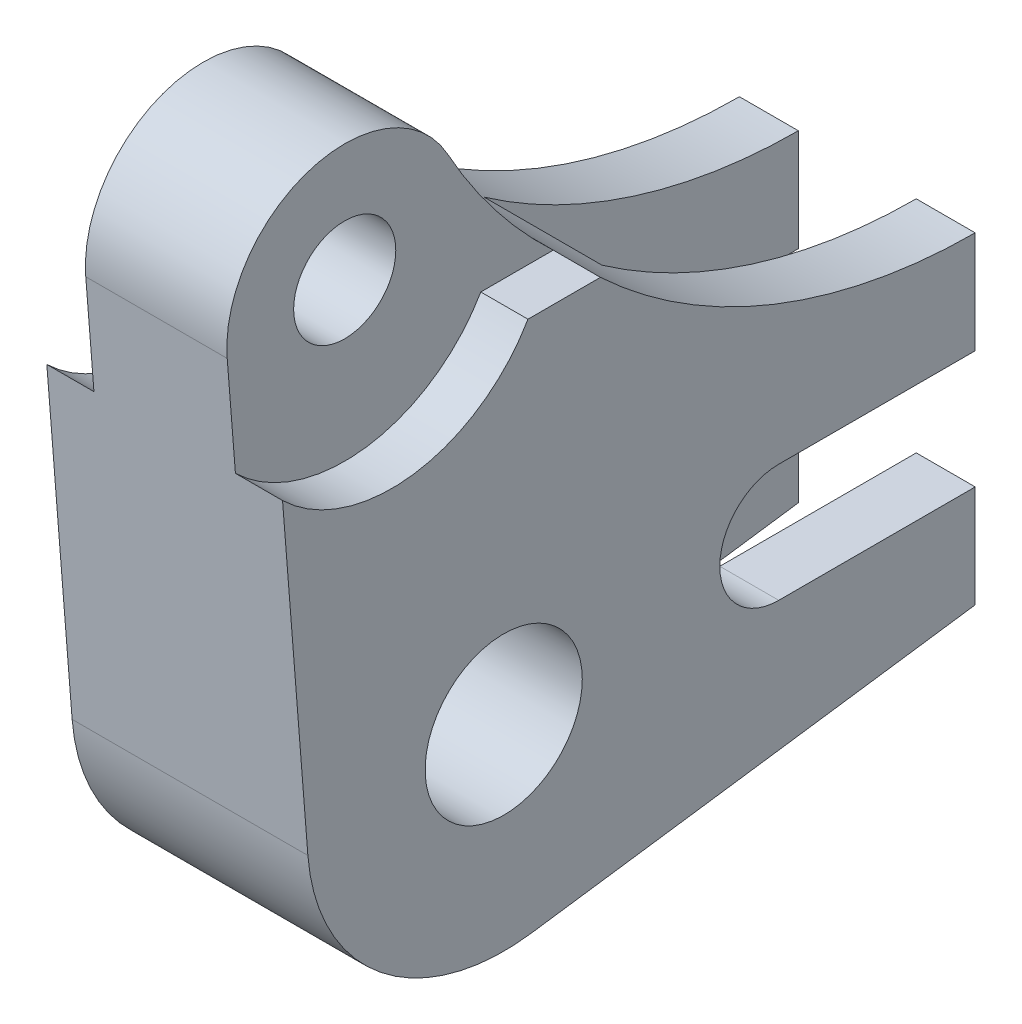
ISO-10303-21;
HEADER;
FILE_DESCRIPTION(('STEP AP214'),'2;1');
FILE_NAME('part.step','',(''),(''),'','','');
FILE_SCHEMA(('AUTOMOTIVE_DESIGN { 1 0 10303 214 1 1 1 1 }'));
ENDSEC;
DATA;
#1=APPLICATION_CONTEXT('core data for automotive mechanical design processes');
#2=APPLICATION_PROTOCOL_DEFINITION('international standard','automotive_design',2000,#1);
#3=PRODUCT_CONTEXT('',#1,'mechanical');
#4=PRODUCT('Part','Part','',(#3));
#5=PRODUCT_RELATED_PRODUCT_CATEGORY('part','',(#4));
#6=PRODUCT_DEFINITION_FORMATION('','',#4);
#7=PRODUCT_DEFINITION_CONTEXT('part definition',#1,'design');
#8=PRODUCT_DEFINITION('design','',#6,#7);
#9=PRODUCT_DEFINITION_SHAPE('','',#8);
#10=(LENGTH_UNIT() NAMED_UNIT(*) SI_UNIT(.MILLI.,.METRE.));
#11=(NAMED_UNIT(*) PLANE_ANGLE_UNIT() SI_UNIT($,.RADIAN.));
#12=(NAMED_UNIT(*) SI_UNIT($,.STERADIAN.) SOLID_ANGLE_UNIT());
#13=UNCERTAINTY_MEASURE_WITH_UNIT(LENGTH_MEASURE(1.E-05),#10,'distance_accuracy_value','');
#14=(GEOMETRIC_REPRESENTATION_CONTEXT(3) GLOBAL_UNCERTAINTY_ASSIGNED_CONTEXT((#13)) GLOBAL_UNIT_ASSIGNED_CONTEXT((#10,
#11,#12)) REPRESENTATION_CONTEXT('',''));
#15=CARTESIAN_POINT('',(0.,0.,0.));
#16=DIRECTION('',(0.,0.,1.));
#17=DIRECTION('',(1.,0.,0.));
#18=AXIS2_PLACEMENT_3D('',#15,#16,#17);
#19=CARTESIAN_POINT('',(15.,-3.81323923082236,-60.));
#20=DIRECTION('',(0.,0.,1.));
#21=DIRECTION('',(1.,0.,0.));
#22=AXIS2_PLACEMENT_3D('',#19,#20,#21);
#23=PLANE('',#22);
#24=DIRECTION('',(0.,-1.,0.));
#25=VECTOR('',#24,1.);
#26=CARTESIAN_POINT('',(7.5,68.1259204458987,-60.));
#27=LINE('',#26,#25);
#28=CARTESIAN_POINT('',(7.5,-3.81323923082236,-60.));
#29=VERTEX_POINT('',#28);
#30=CARTESIAN_POINT('',(7.5,-16.8132392308223,-60.));
#31=VERTEX_POINT('',#30);
#32=EDGE_CURVE('E199',#29,#31,#27,.T.);
#33=ORIENTED_EDGE('',*,*,#32,.F.);
#34=DIRECTION('',(-1.,0.,0.));
#35=VECTOR('',#34,1.);
#36=CARTESIAN_POINT('',(15.,-3.81323923082236,-60.));
#37=LINE('',#36,#35);
#38=CARTESIAN_POINT('',(15.,-3.81323923082236,-60.));
#39=VERTEX_POINT('',#38);
#40=EDGE_CURVE('E361',#39,#29,#37,.T.);
#41=ORIENTED_EDGE('',*,*,#40,.F.);
#42=DIRECTION('',(0.,1.,0.));
#43=VECTOR('',#42,1.);
#44=CARTESIAN_POINT('',(15.,-3.81323923082236,-60.));
#45=LINE('',#44,#43);
#46=CARTESIAN_POINT('',(15.,-16.8132392308224,-60.));
#47=VERTEX_POINT('',#46);
#48=EDGE_CURVE('E296',#47,#39,#45,.T.);
#49=ORIENTED_EDGE('',*,*,#48,.F.);
#50=DIRECTION('',(-1.,0.,0.));
#51=VECTOR('',#50,1.);
#52=CARTESIAN_POINT('',(15.,-16.8132392308224,-60.));
#53=LINE('',#52,#51);
#54=EDGE_CURVE('E370',#47,#31,#53,.T.);
#55=ORIENTED_EDGE('',*,*,#54,.T.);
#56=EDGE_LOOP('',(#33,#41,#49,#55));
#57=FACE_BOUND('',#56,.T.);
#58=ADVANCED_FACE('F39',(#57),#23,.F.);
#59=CARTESIAN_POINT('',(15.,24.1867607691776,-60.));
#60=DIRECTION('',(0.,0.,1.));
#61=DIRECTION('',(0.,-1.,0.));
#62=AXIS2_PLACEMENT_3D('',#59,#60,#61);
#63=PLANE('',#62);
#64=CARTESIAN_POINT('',(7.5,24.1867607691776,-60.));
#65=VERTEX_POINT('',#64);
#66=CARTESIAN_POINT('',(7.5,11.1867607691776,-60.));
#67=VERTEX_POINT('',#66);
#68=EDGE_CURVE('E214',#65,#67,#27,.T.);
#69=ORIENTED_EDGE('',*,*,#68,.F.);
#70=DIRECTION('',(-1.,0.,0.));
#71=VECTOR('',#70,1.);
#72=CARTESIAN_POINT('',(15.,24.1867607691776,-60.));
#73=LINE('',#72,#71);
#74=CARTESIAN_POINT('',(15.,24.1867607691776,-60.));
#75=VERTEX_POINT('',#74);
#76=EDGE_CURVE('E350',#75,#65,#73,.T.);
#77=ORIENTED_EDGE('',*,*,#76,.F.);
#78=DIRECTION('',(0.,1.,0.));
#79=VECTOR('',#78,1.);
#80=CARTESIAN_POINT('',(15.,24.1867607691776,-60.));
#81=LINE('',#80,#79);
#82=CARTESIAN_POINT('',(15.,11.1867607691776,-60.));
#83=VERTEX_POINT('',#82);
#84=EDGE_CURVE('E308',#83,#75,#81,.T.);
#85=ORIENTED_EDGE('',*,*,#84,.F.);
#86=DIRECTION('',(-1.,0.,0.));
#87=VECTOR('',#86,1.);
#88=CARTESIAN_POINT('',(15.,11.1867607691776,-60.));
#89=LINE('',#88,#87);
#90=EDGE_CURVE('E353',#83,#67,#89,.T.);
#91=ORIENTED_EDGE('',*,*,#90,.T.);
#92=EDGE_LOOP('',(#69,#77,#85,#91));
#93=FACE_BOUND('',#92,.T.);
#94=ADVANCED_FACE('F379',(#93),#63,.F.);
#95=CARTESIAN_POINT('',(15.,-16.8132392308224,-60.));
#96=DIRECTION('',(0.,0.990268068741571,0.139173100960059));
#97=DIRECTION('',(0.,-0.139173100960059,0.990268068741571));
#98=AXIS2_PLACEMENT_3D('',#95,#96,#97);
#99=PLANE('',#98);
#100=DIRECTION('',(0.,0.139173100960059,-0.990268068741571));
#101=VECTOR('',#100,1.);
#102=CARTESIAN_POINT('',(-7.5,-16.8132392308224,-60.));
#103=LINE('',#102,#101);
#104=CARTESIAN_POINT('',(-7.49999999999999,-22.4348726189177,-20.));
#105=VERTEX_POINT('',#104);
#106=CARTESIAN_POINT('',(-7.5,-16.8132392308223,-60.));
#107=VERTEX_POINT('',#106);
#108=EDGE_CURVE('E219',#105,#107,#103,.T.);
#109=ORIENTED_EDGE('',*,*,#108,.F.);
#110=DIRECTION('',(-1.,0.,0.));
#111=VECTOR('',#110,1.);
#112=CARTESIAN_POINT('',(15.,-22.4348726189177,-20.));
#113=LINE('',#112,#111);
#114=CARTESIAN_POINT('',(7.50000000000001,-22.4348726189177,-20.));
#115=VERTEX_POINT('',#114);
#116=EDGE_CURVE('E202',#115,#105,#113,.T.);
#117=ORIENTED_EDGE('',*,*,#116,.F.);
#118=DIRECTION('',(0.,-0.139173100960059,0.990268068741571));
#119=VECTOR('',#118,1.);
#120=CARTESIAN_POINT('',(7.5,-16.8132392308224,-60.));
#121=LINE('',#120,#119);
#122=EDGE_CURVE('E197',#31,#115,#121,.T.);
#123=ORIENTED_EDGE('',*,*,#122,.F.);
#124=ORIENTED_EDGE('',*,*,#54,.F.);
#125=DIRECTION('',(0.,0.139173100960059,-0.990268068741571));
#126=VECTOR('',#125,1.);
#127=CARTESIAN_POINT('',(15.,-16.8132392308224,-60.));
#128=LINE('',#127,#126);
#129=CARTESIAN_POINT('',(15.,-24.7567017185393,-3.47932752400147));
#130=VERTEX_POINT('',#129);
#131=EDGE_CURVE('E293',#130,#47,#128,.T.);
#132=ORIENTED_EDGE('',*,*,#131,.F.);
#133=DIRECTION('',(-1.,0.,0.));
#134=VECTOR('',#133,1.);
#135=CARTESIAN_POINT('',(15.,-24.7567017185393,-3.47932752400147));
#136=LINE('',#135,#134);
#137=CARTESIAN_POINT('',(-15.,-24.7567017185393,-3.47932752400147));
#138=VERTEX_POINT('',#137);
#139=EDGE_CURVE('E369',#130,#138,#136,.T.);
#140=ORIENTED_EDGE('',*,*,#139,.T.);
#141=DIRECTION('',(0.,0.139173100960059,-0.990268068741571));
#142=VECTOR('',#141,1.);
#143=CARTESIAN_POINT('',(-15.,-16.8132392308224,-60.));
#144=LINE('',#143,#142);
#145=CARTESIAN_POINT('',(-15.,-16.8132392308224,-60.));
#146=VERTEX_POINT('',#145);
#147=EDGE_CURVE('E316',#138,#146,#144,.T.);
#148=ORIENTED_EDGE('',*,*,#147,.T.);
#149=EDGE_CURVE('E368',#107,#146,#53,.T.);
#150=ORIENTED_EDGE('',*,*,#149,.F.);
#151=EDGE_LOOP('',(#109,#117,#123,#124,#132,#140,#148,#150));
#152=FACE_BOUND('',#151,.T.);
#153=ADVANCED_FACE('F217',(#152),#99,.F.);
#154=CARTESIAN_POINT('',(15.,-3.81323923082236,-35.));
#155=DIRECTION('',(0.,-1.,0.));
#156=DIRECTION('',(0.,0.,-1.));
#157=AXIS2_PLACEMENT_3D('',#154,#155,#156);
#158=PLANE('',#157);
#159=DIRECTION('',(0.,0.,1.));
#160=VECTOR('',#159,1.);
#161=CARTESIAN_POINT('',(-7.5,-3.81323923082236,-35.));
#162=LINE('',#161,#160);
#163=CARTESIAN_POINT('',(-7.5,-3.81323923082236,-60.));
#164=VERTEX_POINT('',#163);
#165=CARTESIAN_POINT('',(-7.5,-3.81323923082236,-35.));
#166=VERTEX_POINT('',#165);
#167=EDGE_CURVE('E226',#164,#166,#162,.T.);
#168=ORIENTED_EDGE('',*,*,#167,.F.);
#169=CARTESIAN_POINT('',(-15.,-3.81323923082236,-60.));
#170=VERTEX_POINT('',#169);
#171=EDGE_CURVE('E362',#164,#170,#37,.T.);
#172=ORIENTED_EDGE('',*,*,#171,.T.);
#173=DIRECTION('',(0.,0.,1.));
#174=VECTOR('',#173,1.);
#175=CARTESIAN_POINT('',(-15.,-3.81323923082236,-35.));
#176=LINE('',#175,#174);
#177=CARTESIAN_POINT('',(-15.,-3.81323923082236,-35.));
#178=VERTEX_POINT('',#177);
#179=EDGE_CURVE('E325',#170,#178,#176,.T.);
#180=ORIENTED_EDGE('',*,*,#179,.T.);
#181=DIRECTION('',(-1.,0.,0.));
#182=VECTOR('',#181,1.);
#183=CARTESIAN_POINT('',(15.,-3.81323923082236,-35.));
#184=LINE('',#183,#182);
#185=EDGE_CURVE('E360',#166,#178,#184,.T.);
#186=ORIENTED_EDGE('',*,*,#185,.F.);
#187=EDGE_LOOP('',(#168,#172,#180,#186));
#188=FACE_BOUND('',#187,.T.);
#189=ADVANCED_FACE('F503',(#188),#158,.F.);
#190=DIRECTION('',(0.,0.,-1.));
#191=VECTOR('',#190,1.);
#192=CARTESIAN_POINT('',(7.5,-3.81323923082236,-35.));
#193=LINE('',#192,#191);
#194=CARTESIAN_POINT('',(7.5,-3.81323923082236,-35.));
#195=VERTEX_POINT('',#194);
#196=EDGE_CURVE('E206',#195,#29,#193,.T.);
#197=ORIENTED_EDGE('',*,*,#196,.F.);
#198=CARTESIAN_POINT('',(15.,-3.81323923082236,-35.));
#199=VERTEX_POINT('',#198);
#200=EDGE_CURVE('E356',#199,#195,#184,.T.);
#201=ORIENTED_EDGE('',*,*,#200,.F.);
#202=DIRECTION('',(0.,0.,1.));
#203=VECTOR('',#202,1.);
#204=CARTESIAN_POINT('',(15.,-3.81323923082236,-35.));
#205=LINE('',#204,#203);
#206=EDGE_CURVE('E299',#39,#199,#205,.T.);
#207=ORIENTED_EDGE('',*,*,#206,.F.);
#208=ORIENTED_EDGE('',*,*,#40,.T.);
#209=EDGE_LOOP('',(#197,#201,#207,#208));
#210=FACE_BOUND('',#209,.T.);
#211=ADVANCED_FACE('F414',(#210),#158,.F.);
#212=CARTESIAN_POINT('',(15.,3.68676076917764,-35.));
#213=DIRECTION('',(-1.,0.,0.));
#214=DIRECTION('',(0.,0.,1.));
#215=AXIS2_PLACEMENT_3D('',#212,#213,#214);
#216=CYLINDRICAL_SURFACE('',#215,7.5);
#217=CARTESIAN_POINT('',(-7.5,3.68676076917764,-35.));
#218=DIRECTION('',(1.,0.,0.));
#219=DIRECTION('',(0.,0.,-1.));
#220=AXIS2_PLACEMENT_3D('',#217,#218,#219);
#221=CIRCLE('',#220,7.5);
#222=CARTESIAN_POINT('',(-7.5,11.1867607691776,-35.));
#223=VERTEX_POINT('',#222);
#224=EDGE_CURVE('E224',#166,#223,#221,.F.);
#225=ORIENTED_EDGE('',*,*,#224,.F.);
#226=ORIENTED_EDGE('',*,*,#185,.T.);
#227=CARTESIAN_POINT('',(-15.,3.68676076917764,-35.));
#228=DIRECTION('',(-1.,0.,0.));
#229=DIRECTION('',(0.,0.,-1.));
#230=AXIS2_PLACEMENT_3D('',#227,#228,#229);
#231=CIRCLE('',#230,7.5);
#232=CARTESIAN_POINT('',(-15.,11.1867607691776,-35.));
#233=VERTEX_POINT('',#232);
#234=EDGE_CURVE('E324',#178,#233,#231,.T.);
#235=ORIENTED_EDGE('',*,*,#234,.T.);
#236=DIRECTION('',(-1.,0.,0.));
#237=VECTOR('',#236,1.);
#238=CARTESIAN_POINT('',(15.,11.1867607691776,-35.));
#239=LINE('',#238,#237);
#240=EDGE_CURVE('E352',#223,#233,#239,.T.);
#241=ORIENTED_EDGE('',*,*,#240,.F.);
#242=EDGE_LOOP('',(#225,#226,#235,#241));
#243=FACE_BOUND('',#242,.T.);
#244=ADVANCED_FACE('F499',(#243),#216,.F.);
#245=CARTESIAN_POINT('',(7.5,3.68676076917764,-35.));
#246=DIRECTION('',(-1.,0.,0.));
#247=DIRECTION('',(0.,0.,1.));
#248=AXIS2_PLACEMENT_3D('',#245,#246,#247);
#249=CIRCLE('',#248,7.5);
#250=CARTESIAN_POINT('',(7.5,11.1867607691776,-35.));
#251=VERTEX_POINT('',#250);
#252=EDGE_CURVE('E398',#251,#195,#249,.F.);
#253=ORIENTED_EDGE('',*,*,#252,.F.);
#254=CARTESIAN_POINT('',(15.,11.1867607691776,-35.));
#255=VERTEX_POINT('',#254);
#256=EDGE_CURVE('E354',#255,#251,#239,.T.);
#257=ORIENTED_EDGE('',*,*,#256,.F.);
#258=CARTESIAN_POINT('',(15.,3.68676076917764,-35.));
#259=DIRECTION('',(-1.,0.,0.));
#260=DIRECTION('',(0.,0.,-1.));
#261=AXIS2_PLACEMENT_3D('',#258,#259,#260);
#262=CIRCLE('',#261,7.5);
#263=EDGE_CURVE('E304',#199,#255,#262,.T.);
#264=ORIENTED_EDGE('',*,*,#263,.F.);
#265=ORIENTED_EDGE('',*,*,#200,.T.);
#266=EDGE_LOOP('',(#253,#257,#264,#265));
#267=FACE_BOUND('',#266,.T.);
#268=ADVANCED_FACE('F500',(#267),#216,.F.);
#269=CARTESIAN_POINT('',(15.,11.1867607691776,-60.));
#270=DIRECTION('',(0.,1.,0.));
#271=DIRECTION('',(0.,0.,1.));
#272=AXIS2_PLACEMENT_3D('',#269,#270,#271);
#273=PLANE('',#272);
#274=DIRECTION('',(0.,0.,-1.));
#275=VECTOR('',#274,1.);
#276=CARTESIAN_POINT('',(-7.5,11.1867607691776,-60.));
#277=LINE('',#276,#275);
#278=CARTESIAN_POINT('',(-7.5,11.1867607691776,-60.));
#279=VERTEX_POINT('',#278);
#280=EDGE_CURVE('E222',#223,#279,#277,.T.);
#281=ORIENTED_EDGE('',*,*,#280,.F.);
#282=ORIENTED_EDGE('',*,*,#240,.T.);
#283=DIRECTION('',(0.,0.,-1.));
#284=VECTOR('',#283,1.);
#285=CARTESIAN_POINT('',(-15.,11.1867607691776,-60.));
#286=LINE('',#285,#284);
#287=CARTESIAN_POINT('',(-15.,11.1867607691776,-60.));
#288=VERTEX_POINT('',#287);
#289=EDGE_CURVE('E327',#233,#288,#286,.T.);
#290=ORIENTED_EDGE('',*,*,#289,.T.);
#291=EDGE_CURVE('E348',#279,#288,#89,.T.);
#292=ORIENTED_EDGE('',*,*,#291,.F.);
#293=EDGE_LOOP('',(#281,#282,#290,#292));
#294=FACE_BOUND('',#293,.T.);
#295=ADVANCED_FACE('F438',(#294),#273,.F.);
#296=DIRECTION('',(0.,0.,1.));
#297=VECTOR('',#296,1.);
#298=CARTESIAN_POINT('',(7.5,11.1867607691776,-60.));
#299=LINE('',#298,#297);
#300=EDGE_CURVE('E400',#67,#251,#299,.T.);
#301=ORIENTED_EDGE('',*,*,#300,.F.);
#302=ORIENTED_EDGE('',*,*,#90,.F.);
#303=DIRECTION('',(0.,0.,-1.));
#304=VECTOR('',#303,1.);
#305=CARTESIAN_POINT('',(15.,11.1867607691776,-60.));
#306=LINE('',#305,#304);
#307=EDGE_CURVE('E301',#255,#83,#306,.T.);
#308=ORIENTED_EDGE('',*,*,#307,.F.);
#309=ORIENTED_EDGE('',*,*,#256,.T.);
#310=EDGE_LOOP('',(#301,#302,#308,#309));
#311=FACE_BOUND('',#310,.T.);
#312=ADVANCED_FACE('F399',(#311),#273,.F.);
#313=CARTESIAN_POINT('',(15.,94.1865039901961,-60.1896021927174));
#314=DIRECTION('',(-1.,0.,0.));
#315=DIRECTION('',(0.,0.,1.));
#316=AXIS2_PLACEMENT_3D('',#313,#314,#315);
#317=CYLINDRICAL_SURFACE('',#316,70.);
#318=CARTESIAN_POINT('',(-7.5,94.1865039901961,-60.1896021927174));
#319=DIRECTION('',(1.,0.,0.));
#320=DIRECTION('',(0.,0.,-1.));
#321=AXIS2_PLACEMENT_3D('',#318,#319,#320);
#322=CIRCLE('',#321,70.);
#323=CARTESIAN_POINT('',(-7.5,24.1867607691776,-60.));
#324=VERTEX_POINT('',#323);
#325=CARTESIAN_POINT('',(-7.49999999999999,36.8733652208779,-20.));
#326=VERTEX_POINT('',#325);
#327=EDGE_CURVE('E11',#324,#326,#322,.F.);
#328=ORIENTED_EDGE('',*,*,#327,.F.);
#329=CARTESIAN_POINT('',(-15.,24.1867607691776,-60.));
#330=VERTEX_POINT('',#329);
#331=EDGE_CURVE('E347',#324,#330,#73,.T.);
#332=ORIENTED_EDGE('',*,*,#331,.T.);
#333=CARTESIAN_POINT('',(-15.,94.1865039901961,-60.1896021927174));
#334=DIRECTION('',(-1.,0.,0.));
#335=DIRECTION('',(0.,0.,-1.));
#336=AXIS2_PLACEMENT_3D('',#333,#334,#335);
#337=CIRCLE('',#336,70.);
#338=CARTESIAN_POINT('',(-15.,43.1259204458988,-12.3062354761233));
#339=VERTEX_POINT('',#338);
#340=EDGE_CURVE('E331',#330,#339,#337,.T.);
#341=ORIENTED_EDGE('',*,*,#340,.T.);
#342=DIRECTION('',(-1.,0.,0.));
#343=VECTOR('',#342,1.);
#344=CARTESIAN_POINT('',(-9.,43.1259204458988,-12.3062354761233));
#345=LINE('',#344,#343);
#346=CARTESIAN_POINT('',(-9.,43.1259204458988,-12.3062354761233));
#347=VERTEX_POINT('',#346);
#348=EDGE_CURVE('E255',#347,#339,#345,.T.);
#349=ORIENTED_EDGE('',*,*,#348,.F.);
#350=CARTESIAN_POINT('',(-9.,94.1865039901961,-60.1896021927174));
#351=DIRECTION('',(-1.,0.,0.));
#352=DIRECTION('',(0.,0.,-1.));
#353=AXIS2_PLACEMENT_3D('',#350,#351,#352);
#354=CIRCLE('',#353,70.);
#355=CARTESIAN_POINT('',(-9.,60.3719057772453,1.10128577357586));
#356=VERTEX_POINT('',#355);
#357=EDGE_CURVE('E65',#347,#356,#354,.T.);
#358=ORIENTED_EDGE('',*,*,#357,.T.);
#359=DIRECTION('',(-1.,0.,0.));
#360=VECTOR('',#359,1.);
#361=CARTESIAN_POINT('',(15.,60.3719057772453,1.10128577357586));
#362=LINE('',#361,#360);
#363=CARTESIAN_POINT('',(9.,60.3719057772453,1.10128577357586));
#364=VERTEX_POINT('',#363);
#365=EDGE_CURVE('E345',#364,#356,#362,.T.);
#366=ORIENTED_EDGE('',*,*,#365,.F.);
#367=CARTESIAN_POINT('',(9.,94.1865039901961,-60.1896021927174));
#368=DIRECTION('',(-1.,0.,0.));
#369=DIRECTION('',(0.,0.,-1.));
#370=AXIS2_PLACEMENT_3D('',#367,#368,#369);
#371=CIRCLE('',#370,70.);
#372=CARTESIAN_POINT('',(9.,43.1259204458988,-12.3062354761233));
#373=VERTEX_POINT('',#372);
#374=EDGE_CURVE('E268',#373,#364,#371,.T.);
#375=ORIENTED_EDGE('',*,*,#374,.F.);
#376=DIRECTION('',(1.,0.,0.));
#377=VECTOR('',#376,1.);
#378=CARTESIAN_POINT('',(9.,43.1259204458988,-12.3062354761233));
#379=LINE('',#378,#377);
#380=CARTESIAN_POINT('',(15.,43.1259204458988,-12.3062354761233));
#381=VERTEX_POINT('',#380);
#382=EDGE_CURVE('E283',#373,#381,#379,.T.);
#383=ORIENTED_EDGE('',*,*,#382,.T.);
#384=CARTESIAN_POINT('',(15.,94.1865039901961,-60.1896021927174));
#385=DIRECTION('',(-1.,0.,0.));
#386=DIRECTION('',(0.,0.,-1.));
#387=AXIS2_PLACEMENT_3D('',#384,#385,#386);
#388=CIRCLE('',#387,70.);
#389=EDGE_CURVE('E306',#75,#381,#388,.T.);
#390=ORIENTED_EDGE('',*,*,#389,.F.);
#391=ORIENTED_EDGE('',*,*,#76,.T.);
#392=CARTESIAN_POINT('',(7.5,94.1865039901961,-60.1896021927174));
#393=DIRECTION('',(-1.,0.,0.));
#394=DIRECTION('',(0.,0.,1.));
#395=AXIS2_PLACEMENT_3D('',#392,#393,#394);
#396=CIRCLE('',#395,70.);
#397=CARTESIAN_POINT('',(7.50000000000001,36.8733652208779,-20.));
#398=VERTEX_POINT('',#397);
#399=EDGE_CURVE('E375',#398,#65,#396,.F.);
#400=ORIENTED_EDGE('',*,*,#399,.F.);
#401=DIRECTION('',(-1.,0.,0.));
#402=VECTOR('',#401,1.);
#403=CARTESIAN_POINT('',(15.,36.8733652208779,-20.));
#404=LINE('',#403,#402);
#405=EDGE_CURVE('E50',#326,#398,#404,.F.);
#406=ORIENTED_EDGE('',*,*,#405,.F.);
#407=EDGE_LOOP('',(#328,#332,#341,#349,#358,#366,#375,#383,#390,#391,#400,#406));
#408=FACE_BOUND('',#407,.T.);
#409=ADVANCED_FACE('F387',(#408),#317,.F.);
#410=CARTESIAN_POINT('',(15.,53.1259204458987,14.2350474806387));
#411=DIRECTION('',(-1.,0.,0.));
#412=DIRECTION('',(0.,0.,1.));
#413=AXIS2_PLACEMENT_3D('',#410,#411,#412);
#414=CYLINDRICAL_SURFACE('',#413,6.5);
#415=CARTESIAN_POINT('',(9.,53.1259204458987,14.2350474806387));
#416=DIRECTION('',(1.,0.,0.));
#417=DIRECTION('',(0.,0.,-1.));
#418=AXIS2_PLACEMENT_3D('',#415,#416,#417);
#419=CIRCLE('',#418,6.5);
#420=CARTESIAN_POINT('',(9.,53.1259204458987,7.73504748063869));
#421=VERTEX_POINT('',#420);
#422=EDGE_CURVE('E278',#421,#421,#419,.T.);
#423=ORIENTED_EDGE('',*,*,#422,.T.);
#424=EDGE_LOOP('',(#423));
#425=FACE_BOUND('',#424,.T.);
#426=CARTESIAN_POINT('',(-9.,53.1259204458987,14.2350474806387));
#427=DIRECTION('',(-1.,0.,0.));
#428=DIRECTION('',(0.,0.,1.));
#429=AXIS2_PLACEMENT_3D('',#426,#427,#428);
#430=CIRCLE('',#429,6.5);
#431=CARTESIAN_POINT('',(-9.,53.1259204458987,20.7350474806387));
#432=VERTEX_POINT('',#431);
#433=EDGE_CURVE('E251',#432,#432,#430,.T.);
#434=ORIENTED_EDGE('',*,*,#433,.T.);
#435=EDGE_LOOP('',(#434));
#436=FACE_BOUND('',#435,.T.);
#437=ADVANCED_FACE('F488',(#425,#436),#414,.F.);
#438=CARTESIAN_POINT('',(-15.,0.,0.));
#439=DIRECTION('',(1.,0.,0.));
#440=DIRECTION('',(0.,0.,-1.));
#441=AXIS2_PLACEMENT_3D('',#438,#439,#440);
#442=PLANE('',#441);
#443=CARTESIAN_POINT('',(-15.,0.,0.));
#444=DIRECTION('',(1.,0.,0.));
#445=DIRECTION('',(0.,0.,-1.));
#446=AXIS2_PLACEMENT_3D('',#443,#444,#445);
#447=CIRCLE('',#446,10.);
#448=CARTESIAN_POINT('',(-15.,0.,-10.));
#449=VERTEX_POINT('',#448);
#450=EDGE_CURVE('E286',#449,#449,#447,.T.);
#451=ORIENTED_EDGE('',*,*,#450,.T.);
#452=EDGE_LOOP('',(#451));
#453=FACE_BOUND('',#452,.T.);
#454=DIRECTION('',(0.,-0.996883943195047,-0.0788822147248336));
#455=VECTOR('',#454,1.);
#456=CARTESIAN_POINT('',(-15.,-1.97205536812084,24.9220985798762));
#457=LINE('',#456,#455);
#458=CARTESIAN_POINT('',(-15.,38.7551522265886,28.1447930134248));
#459=VERTEX_POINT('',#458);
#460=CARTESIAN_POINT('',(-15.,-1.97205536812084,24.9220985798762));
#461=VERTEX_POINT('',#460);
#462=EDGE_CURVE('E298',#459,#461,#457,.T.);
#463=ORIENTED_EDGE('',*,*,#462,.F.);
#464=CARTESIAN_POINT('',(-15.,53.1259204458987,14.2350474806387));
#465=DIRECTION('',(1.,0.,0.));
#466=DIRECTION('',(0.,0.,-1.));
#467=AXIS2_PLACEMENT_3D('',#464,#465,#466);
#468=CIRCLE('',#467,20.);
#469=CARTESIAN_POINT('',(-15.,43.1259204458987,-3.08546059505009));
#470=VERTEX_POINT('',#469);
#471=EDGE_CURVE('E232',#459,#470,#468,.T.);
#472=ORIENTED_EDGE('',*,*,#471,.T.);
#473=DIRECTION('',(0.,0.,-1.));
#474=VECTOR('',#473,1.);
#475=CARTESIAN_POINT('',(-15.,43.1259204458987,-3.08546059505009));
#476=LINE('',#475,#474);
#477=EDGE_CURVE('E237',#470,#339,#476,.T.);
#478=ORIENTED_EDGE('',*,*,#477,.T.);
#479=ORIENTED_EDGE('',*,*,#340,.F.);
#480=DIRECTION('',(0.,1.,0.));
#481=VECTOR('',#480,1.);
#482=CARTESIAN_POINT('',(-15.,24.1867607691776,-60.));
#483=LINE('',#482,#481);
#484=EDGE_CURVE('E332',#288,#330,#483,.T.);
#485=ORIENTED_EDGE('',*,*,#484,.F.);
#486=ORIENTED_EDGE('',*,*,#289,.F.);
#487=ORIENTED_EDGE('',*,*,#234,.F.);
#488=ORIENTED_EDGE('',*,*,#179,.F.);
#489=DIRECTION('',(0.,1.,0.));
#490=VECTOR('',#489,1.);
#491=CARTESIAN_POINT('',(-15.,-3.81323923082236,-60.));
#492=LINE('',#491,#490);
#493=EDGE_CURVE('E317',#146,#170,#492,.T.);
#494=ORIENTED_EDGE('',*,*,#493,.F.);
#495=ORIENTED_EDGE('',*,*,#147,.F.);
#496=CARTESIAN_POINT('',(-15.,0.,0.));
#497=DIRECTION('',(1.,0.,0.));
#498=DIRECTION('',(0.,0.,-1.));
#499=AXIS2_PLACEMENT_3D('',#496,#497,#498);
#500=CIRCLE('',#499,25.);
#501=EDGE_CURVE('E290',#461,#138,#500,.T.);
#502=ORIENTED_EDGE('',*,*,#501,.F.);
#503=EDGE_LOOP('',(#463,#472,#478,#479,#485,#486,#487,#488,#494,#495,#502));
#504=FACE_BOUND('',#503,.T.);
#505=ADVANCED_FACE('F423',(#453,#504),#442,.F.);
#506=CARTESIAN_POINT('',(15.,53.1259204458987,14.2350474806387));
#507=DIRECTION('',(-1.,0.,0.));
#508=DIRECTION('',(0.,0.,1.));
#509=AXIS2_PLACEMENT_3D('',#506,#507,#508);
#510=CYLINDRICAL_SURFACE('',#509,15.);
#511=ORIENTED_EDGE('',*,*,#365,.T.);
#512=CARTESIAN_POINT('',(-9.,53.1259204458987,14.2350474806387));
#513=DIRECTION('',(1.,0.,0.));
#514=DIRECTION('',(0.,0.,-1.));
#515=AXIS2_PLACEMENT_3D('',#512,#513,#514);
#516=CIRCLE('',#515,15.);
#517=CARTESIAN_POINT('',(-9.,51.9426872250262,29.1883066285644));
#518=VERTEX_POINT('',#517);
#519=EDGE_CURVE('E239',#356,#518,#516,.T.);
#520=ORIENTED_EDGE('',*,*,#519,.T.);
#521=DIRECTION('',(-1.,0.,0.));
#522=VECTOR('',#521,1.);
#523=CARTESIAN_POINT('',(15.,51.9426872250262,29.1883066285644));
#524=LINE('',#523,#522);
#525=CARTESIAN_POINT('',(9.,51.9426872250262,29.1883066285644));
#526=VERTEX_POINT('',#525);
#527=EDGE_CURVE('E339',#526,#518,#524,.T.);
#528=ORIENTED_EDGE('',*,*,#527,.F.);
#529=CARTESIAN_POINT('',(9.,53.1259204458987,14.2350474806387));
#530=DIRECTION('',(1.,0.,0.));
#531=DIRECTION('',(0.,0.,-1.));
#532=AXIS2_PLACEMENT_3D('',#529,#530,#531);
#533=CIRCLE('',#532,15.);
#534=EDGE_CURVE('E269',#364,#526,#533,.T.);
#535=ORIENTED_EDGE('',*,*,#534,.F.);
#536=EDGE_LOOP('',(#511,#520,#528,#535));
#537=FACE_BOUND('',#536,.T.);
#538=ADVANCED_FACE('F481',(#537),#510,.T.);
#539=CARTESIAN_POINT('',(15.,-1.97205536812084,24.9220985798762));
#540=DIRECTION('',(0.,0.0788822147248336,-0.996883943195047));
#541=DIRECTION('',(0.,0.996883943195047,0.0788822147248336));
#542=AXIS2_PLACEMENT_3D('',#539,#540,#541);
#543=PLANE('',#542);
#544=DIRECTION('',(0.,-0.996883943195047,-0.0788822147248336));
#545=VECTOR('',#544,1.);
#546=CARTESIAN_POINT('',(-9.,51.9426872250262,29.1883066285644));
#547=LINE('',#546,#545);
#548=CARTESIAN_POINT('',(-9.,38.7551522265886,28.1447930134248));
#549=VERTEX_POINT('',#548);
#550=EDGE_CURVE('E233',#518,#549,#547,.T.);
#551=ORIENTED_EDGE('',*,*,#550,.T.);
#552=DIRECTION('',(-1.,0.,0.));
#553=VECTOR('',#552,1.);
#554=CARTESIAN_POINT('',(-9.,38.7551522265886,28.1447930134248));
#555=LINE('',#554,#553);
#556=EDGE_CURVE('E244',#549,#459,#555,.T.);
#557=ORIENTED_EDGE('',*,*,#556,.T.);
#558=ORIENTED_EDGE('',*,*,#462,.T.);
#559=DIRECTION('',(-1.,0.,0.));
#560=VECTOR('',#559,1.);
#561=CARTESIAN_POINT('',(15.,-1.97205536812084,24.9220985798762));
#562=LINE('',#561,#560);
#563=CARTESIAN_POINT('',(15.,-1.97205536812084,24.9220985798762));
#564=VERTEX_POINT('',#563);
#565=EDGE_CURVE('E311',#564,#461,#562,.T.);
#566=ORIENTED_EDGE('',*,*,#565,.F.);
#567=DIRECTION('',(0.,-0.996883943195047,-0.0788822147248336));
#568=VECTOR('',#567,1.);
#569=CARTESIAN_POINT('',(15.,-1.97205536812084,24.9220985798762));
#570=LINE('',#569,#568);
#571=CARTESIAN_POINT('',(15.,38.7551522265886,28.1447930134248));
#572=VERTEX_POINT('',#571);
#573=EDGE_CURVE('E313',#572,#564,#570,.T.);
#574=ORIENTED_EDGE('',*,*,#573,.F.);
#575=DIRECTION('',(1.,0.,0.));
#576=VECTOR('',#575,1.);
#577=CARTESIAN_POINT('',(9.,38.7551522265886,28.1447930134248));
#578=LINE('',#577,#576);
#579=CARTESIAN_POINT('',(9.,38.7551522265886,28.1447930134248));
#580=VERTEX_POINT('',#579);
#581=EDGE_CURVE('E279',#580,#572,#578,.T.);
#582=ORIENTED_EDGE('',*,*,#581,.F.);
#583=DIRECTION('',(0.,-0.996883943195047,-0.0788822147248336));
#584=VECTOR('',#583,1.);
#585=CARTESIAN_POINT('',(9.,51.9426872250262,29.1883066285644));
#586=LINE('',#585,#584);
#587=EDGE_CURVE('E275',#526,#580,#586,.T.);
#588=ORIENTED_EDGE('',*,*,#587,.F.);
#589=ORIENTED_EDGE('',*,*,#527,.T.);
#590=EDGE_LOOP('',(#551,#557,#558,#566,#574,#582,#588,#589));
#591=FACE_BOUND('',#590,.T.);
#592=ADVANCED_FACE('F474',(#591),#543,.F.);
#593=CARTESIAN_POINT('',(15.,0.,0.));
#594=DIRECTION('',(1.,0.,0.));
#595=DIRECTION('',(0.,0.,-1.));
#596=AXIS2_PLACEMENT_3D('',#593,#594,#595);
#597=PLANE('',#596);
#598=CARTESIAN_POINT('',(15.,53.1259204458987,14.2350474806387));
#599=DIRECTION('',(1.,0.,0.));
#600=DIRECTION('',(0.,0.,-1.));
#601=AXIS2_PLACEMENT_3D('',#598,#599,#600);
#602=CIRCLE('',#601,20.);
#603=CARTESIAN_POINT('',(15.,43.1259204458987,-3.08546059505009));
#604=VERTEX_POINT('',#603);
#605=EDGE_CURVE('E257',#572,#604,#602,.T.);
#606=ORIENTED_EDGE('',*,*,#605,.F.);
#607=ORIENTED_EDGE('',*,*,#573,.T.);
#608=CARTESIAN_POINT('',(15.,0.,0.));
#609=DIRECTION('',(1.,0.,0.));
#610=DIRECTION('',(0.,0.,-1.));
#611=AXIS2_PLACEMENT_3D('',#608,#609,#610);
#612=CIRCLE('',#611,25.);
#613=EDGE_CURVE('E295',#564,#130,#612,.T.);
#614=ORIENTED_EDGE('',*,*,#613,.T.);
#615=ORIENTED_EDGE('',*,*,#131,.T.);
#616=ORIENTED_EDGE('',*,*,#48,.T.);
#617=ORIENTED_EDGE('',*,*,#206,.T.);
#618=ORIENTED_EDGE('',*,*,#263,.T.);
#619=ORIENTED_EDGE('',*,*,#307,.T.);
#620=ORIENTED_EDGE('',*,*,#84,.T.);
#621=ORIENTED_EDGE('',*,*,#389,.T.);
#622=DIRECTION('',(0.,0.,-1.));
#623=VECTOR('',#622,1.);
#624=CARTESIAN_POINT('',(15.,43.1259204458987,-3.08546059505009));
#625=LINE('',#624,#623);
#626=EDGE_CURVE('E264',#604,#381,#625,.T.);
#627=ORIENTED_EDGE('',*,*,#626,.F.);
#628=EDGE_LOOP('',(#606,#607,#614,#615,#616,#617,#618,#619,#620,#621,#627));
#629=FACE_BOUND('',#628,.T.);
#630=CARTESIAN_POINT('',(15.,0.,0.));
#631=DIRECTION('',(1.,0.,0.));
#632=DIRECTION('',(0.,0.,-1.));
#633=AXIS2_PLACEMENT_3D('',#630,#631,#632);
#634=CIRCLE('',#633,10.);
#635=CARTESIAN_POINT('',(15.,0.,-10.));
#636=VERTEX_POINT('',#635);
#637=EDGE_CURVE('E284',#636,#636,#634,.T.);
#638=ORIENTED_EDGE('',*,*,#637,.F.);
#639=EDGE_LOOP('',(#638));
#640=FACE_BOUND('',#639,.T.);
#641=ADVANCED_FACE('F393',(#629,#640),#597,.T.);
#642=CARTESIAN_POINT('',(15.,0.,0.));
#643=DIRECTION('',(-1.,0.,0.));
#644=DIRECTION('',(0.,0.,1.));
#645=AXIS2_PLACEMENT_3D('',#642,#643,#644);
#646=CYLINDRICAL_SURFACE('',#645,25.);
#647=ORIENTED_EDGE('',*,*,#501,.T.);
#648=ORIENTED_EDGE('',*,*,#139,.F.);
#649=ORIENTED_EDGE('',*,*,#613,.F.);
#650=ORIENTED_EDGE('',*,*,#565,.T.);
#651=EDGE_LOOP('',(#647,#648,#649,#650));
#652=FACE_BOUND('',#651,.T.);
#653=ADVANCED_FACE('F41',(#652),#646,.T.);
#654=ORIENTED_EDGE('',*,*,#171,.F.);
#655=DIRECTION('',(0.,-1.,0.));
#656=VECTOR('',#655,1.);
#657=CARTESIAN_POINT('',(-7.5,68.1259204458987,-60.));
#658=LINE('',#657,#656);
#659=EDGE_CURVE('E428',#164,#107,#658,.T.);
#660=ORIENTED_EDGE('',*,*,#659,.T.);
#661=ORIENTED_EDGE('',*,*,#149,.T.);
#662=ORIENTED_EDGE('',*,*,#493,.T.);
#663=EDGE_LOOP('',(#654,#660,#661,#662));
#664=FACE_BOUND('',#663,.T.);
#665=ADVANCED_FACE('F426',(#664),#23,.F.);
#666=ORIENTED_EDGE('',*,*,#331,.F.);
#667=EDGE_CURVE('E412',#324,#279,#658,.T.);
#668=ORIENTED_EDGE('',*,*,#667,.T.);
#669=ORIENTED_EDGE('',*,*,#291,.T.);
#670=ORIENTED_EDGE('',*,*,#484,.T.);
#671=EDGE_LOOP('',(#666,#668,#669,#670));
#672=FACE_BOUND('',#671,.T.);
#673=ADVANCED_FACE('F436',(#672),#63,.F.);
#674=CARTESIAN_POINT('',(15.,0.,0.));
#675=DIRECTION('',(-1.,0.,0.));
#676=DIRECTION('',(0.,0.,1.));
#677=AXIS2_PLACEMENT_3D('',#674,#675,#676);
#678=CYLINDRICAL_SURFACE('',#677,10.);
#679=ORIENTED_EDGE('',*,*,#637,.T.);
#680=EDGE_LOOP('',(#679));
#681=FACE_BOUND('',#680,.T.);
#682=ORIENTED_EDGE('',*,*,#450,.F.);
#683=EDGE_LOOP('',(#682));
#684=FACE_BOUND('',#683,.T.);
#685=ADVANCED_FACE('F466',(#681,#684),#678,.F.);
#686=CARTESIAN_POINT('',(9.,53.1259204458987,14.2350474806387));
#687=DIRECTION('',(1.,0.,0.));
#688=DIRECTION('',(0.,0.,-1.));
#689=AXIS2_PLACEMENT_3D('',#686,#687,#688);
#690=CYLINDRICAL_SURFACE('',#689,20.);
#691=ORIENTED_EDGE('',*,*,#605,.T.);
#692=DIRECTION('',(1.,0.,0.));
#693=VECTOR('',#692,1.);
#694=CARTESIAN_POINT('',(9.,43.1259204458987,-3.08546059505009));
#695=LINE('',#694,#693);
#696=CARTESIAN_POINT('',(9.,43.1259204458987,-3.08546059505009));
#697=VERTEX_POINT('',#696);
#698=EDGE_CURVE('E273',#697,#604,#695,.T.);
#699=ORIENTED_EDGE('',*,*,#698,.F.);
#700=CARTESIAN_POINT('',(9.,53.1259204458987,14.2350474806387));
#701=DIRECTION('',(1.,0.,0.));
#702=DIRECTION('',(0.,0.,-1.));
#703=AXIS2_PLACEMENT_3D('',#700,#701,#702);
#704=CIRCLE('',#703,20.);
#705=EDGE_CURVE('E261',#580,#697,#704,.T.);
#706=ORIENTED_EDGE('',*,*,#705,.F.);
#707=ORIENTED_EDGE('',*,*,#581,.T.);
#708=EDGE_LOOP('',(#691,#699,#706,#707));
#709=FACE_BOUND('',#708,.T.);
#710=ADVANCED_FACE('F638',(#709),#690,.F.);
#711=CARTESIAN_POINT('',(9.,43.1259204458987,-3.08546059505009));
#712=DIRECTION('',(0.,-1.,0.));
#713=DIRECTION('',(0.,0.,-1.));
#714=AXIS2_PLACEMENT_3D('',#711,#712,#713);
#715=PLANE('',#714);
#716=ORIENTED_EDGE('',*,*,#626,.T.);
#717=ORIENTED_EDGE('',*,*,#382,.F.);
#718=DIRECTION('',(0.,0.,-1.));
#719=VECTOR('',#718,1.);
#720=CARTESIAN_POINT('',(9.,43.1259204458987,-3.08546059505009));
#721=LINE('',#720,#719);
#722=EDGE_CURVE('E262',#697,#373,#721,.T.);
#723=ORIENTED_EDGE('',*,*,#722,.F.);
#724=ORIENTED_EDGE('',*,*,#698,.T.);
#725=EDGE_LOOP('',(#716,#717,#723,#724));
#726=FACE_BOUND('',#725,.T.);
#727=ADVANCED_FACE('F628',(#726),#715,.F.);
#728=CARTESIAN_POINT('',(9.,53.1259204458987,14.2350474806387));
#729=DIRECTION('',(1.,0.,0.));
#730=DIRECTION('',(0.,0.,-1.));
#731=AXIS2_PLACEMENT_3D('',#728,#729,#730);
#732=PLANE('',#731);
#733=ORIENTED_EDGE('',*,*,#422,.F.);
#734=EDGE_LOOP('',(#733));
#735=FACE_BOUND('',#734,.T.);
#736=ORIENTED_EDGE('',*,*,#705,.T.);
#737=ORIENTED_EDGE('',*,*,#722,.T.);
#738=ORIENTED_EDGE('',*,*,#374,.T.);
#739=ORIENTED_EDGE('',*,*,#534,.T.);
#740=ORIENTED_EDGE('',*,*,#587,.T.);
#741=EDGE_LOOP('',(#736,#737,#738,#739,#740));
#742=FACE_BOUND('',#741,.T.);
#743=ADVANCED_FACE('F602',(#735,#742),#732,.T.);
#744=CARTESIAN_POINT('',(-9.,53.1259204458987,14.2350474806387));
#745=DIRECTION('',(-1.,0.,0.));
#746=DIRECTION('',(0.,0.,1.));
#747=AXIS2_PLACEMENT_3D('',#744,#745,#746);
#748=CYLINDRICAL_SURFACE('',#747,20.);
#749=ORIENTED_EDGE('',*,*,#471,.F.);
#750=ORIENTED_EDGE('',*,*,#556,.F.);
#751=CARTESIAN_POINT('',(-9.,53.1259204458987,14.2350474806387));
#752=DIRECTION('',(1.,0.,0.));
#753=DIRECTION('',(0.,0.,-1.));
#754=AXIS2_PLACEMENT_3D('',#751,#752,#753);
#755=CIRCLE('',#754,20.);
#756=CARTESIAN_POINT('',(-9.,43.1259204458987,-3.08546059505009));
#757=VERTEX_POINT('',#756);
#758=EDGE_CURVE('E234',#549,#757,#755,.T.);
#759=ORIENTED_EDGE('',*,*,#758,.T.);
#760=DIRECTION('',(-1.,0.,0.));
#761=VECTOR('',#760,1.);
#762=CARTESIAN_POINT('',(-9.,43.1259204458987,-3.08546059505009));
#763=LINE('',#762,#761);
#764=EDGE_CURVE('E248',#757,#470,#763,.T.);
#765=ORIENTED_EDGE('',*,*,#764,.T.);
#766=EDGE_LOOP('',(#749,#750,#759,#765));
#767=FACE_BOUND('',#766,.T.);
#768=ADVANCED_FACE('F593',(#767),#748,.F.);
#769=CARTESIAN_POINT('',(-9.,43.1259204458987,-3.08546059505009));
#770=DIRECTION('',(0.,1.,0.));
#771=DIRECTION('',(0.,0.,1.));
#772=AXIS2_PLACEMENT_3D('',#769,#770,#771);
#773=PLANE('',#772);
#774=ORIENTED_EDGE('',*,*,#477,.F.);
#775=ORIENTED_EDGE('',*,*,#764,.F.);
#776=DIRECTION('',(0.,0.,-1.));
#777=VECTOR('',#776,1.);
#778=CARTESIAN_POINT('',(-9.,43.1259204458987,-3.08546059505009));
#779=LINE('',#778,#777);
#780=EDGE_CURVE('E241',#757,#347,#779,.T.);
#781=ORIENTED_EDGE('',*,*,#780,.T.);
#782=ORIENTED_EDGE('',*,*,#348,.T.);
#783=EDGE_LOOP('',(#774,#775,#781,#782));
#784=FACE_BOUND('',#783,.T.);
#785=ADVANCED_FACE('F453',(#784),#773,.T.);
#786=CARTESIAN_POINT('',(-9.,53.1259204458987,14.2350474806387));
#787=DIRECTION('',(-1.,0.,0.));
#788=DIRECTION('',(0.,0.,-1.));
#789=AXIS2_PLACEMENT_3D('',#786,#787,#788);
#790=PLANE('',#789);
#791=ORIENTED_EDGE('',*,*,#433,.F.);
#792=EDGE_LOOP('',(#791));
#793=FACE_BOUND('',#792,.T.);
#794=ORIENTED_EDGE('',*,*,#758,.F.);
#795=ORIENTED_EDGE('',*,*,#550,.F.);
#796=ORIENTED_EDGE('',*,*,#519,.F.);
#797=ORIENTED_EDGE('',*,*,#357,.F.);
#798=ORIENTED_EDGE('',*,*,#780,.F.);
#799=EDGE_LOOP('',(#794,#795,#796,#797,#798));
#800=FACE_BOUND('',#799,.T.);
#801=ADVANCED_FACE('F450',(#793,#800),#790,.T.);
#802=CARTESIAN_POINT('',(-7.5,68.1259204458987,-60.));
#803=DIRECTION('',(1.,0.,0.));
#804=DIRECTION('',(0.,0.,-1.));
#805=AXIS2_PLACEMENT_3D('',#802,#803,#804);
#806=PLANE('',#805);
#807=ORIENTED_EDGE('',*,*,#108,.T.);
#808=ORIENTED_EDGE('',*,*,#659,.F.);
#809=ORIENTED_EDGE('',*,*,#167,.T.);
#810=ORIENTED_EDGE('',*,*,#224,.T.);
#811=ORIENTED_EDGE('',*,*,#280,.T.);
#812=ORIENTED_EDGE('',*,*,#667,.F.);
#813=ORIENTED_EDGE('',*,*,#327,.T.);
#814=DIRECTION('',(0.,-1.,0.));
#815=VECTOR('',#814,1.);
#816=CARTESIAN_POINT('',(-7.49999999999999,68.1259204458987,-20.));
#817=LINE('',#816,#815);
#818=EDGE_CURVE('E212',#326,#105,#817,.T.);
#819=ORIENTED_EDGE('',*,*,#818,.T.);
#820=EDGE_LOOP('',(#807,#808,#809,#810,#811,#812,#813,#819));
#821=FACE_BOUND('',#820,.T.);
#822=ADVANCED_FACE('F443',(#821),#806,.T.);
#823=CARTESIAN_POINT('',(-7.49999999999999,68.1259204458987,-20.));
#824=DIRECTION('',(0.,0.,-1.));
#825=DIRECTION('',(-1.,0.,0.));
#826=AXIS2_PLACEMENT_3D('',#823,#824,#825);
#827=PLANE('',#826);
#828=ORIENTED_EDGE('',*,*,#116,.T.);
#829=ORIENTED_EDGE('',*,*,#818,.F.);
#830=ORIENTED_EDGE('',*,*,#405,.T.);
#831=DIRECTION('',(0.,-1.,0.));
#832=VECTOR('',#831,1.);
#833=CARTESIAN_POINT('',(7.50000000000001,68.1259204458987,-20.));
#834=LINE('',#833,#832);
#835=EDGE_CURVE('E53',#398,#115,#834,.T.);
#836=ORIENTED_EDGE('',*,*,#835,.T.);
#837=EDGE_LOOP('',(#828,#829,#830,#836));
#838=FACE_BOUND('',#837,.T.);
#839=ADVANCED_FACE('F207',(#838),#827,.T.);
#840=CARTESIAN_POINT('',(7.5,68.1259204458987,-60.));
#841=DIRECTION('',(-1.,0.,0.));
#842=DIRECTION('',(0.,0.,1.));
#843=AXIS2_PLACEMENT_3D('',#840,#841,#842);
#844=PLANE('',#843);
#845=ORIENTED_EDGE('',*,*,#122,.T.);
#846=ORIENTED_EDGE('',*,*,#835,.F.);
#847=ORIENTED_EDGE('',*,*,#399,.T.);
#848=ORIENTED_EDGE('',*,*,#68,.T.);
#849=ORIENTED_EDGE('',*,*,#300,.T.);
#850=ORIENTED_EDGE('',*,*,#252,.T.);
#851=ORIENTED_EDGE('',*,*,#196,.T.);
#852=ORIENTED_EDGE('',*,*,#32,.T.);
#853=EDGE_LOOP('',(#845,#846,#847,#848,#849,#850,#851,#852));
#854=FACE_BOUND('',#853,.T.);
#855=ADVANCED_FACE('F196',(#854),#844,.T.);
#856=CLOSED_SHELL('',(#58,#94,#153,#189,#211,#244,#268,#295,#312,#409,#437,#505,#538,#592,#641,
#653,#665,#673,#685,#710,#727,#743,#768,#785,#801,#822,#839,#855));
#857=MANIFOLD_SOLID_BREP('B2',#856);
#858=ADVANCED_BREP_SHAPE_REPRESENTATION('',(#18,#857),#14);
#859=SHAPE_DEFINITION_REPRESENTATION(#9,#858);
ENDSEC;
END-ISO-10303-21;
